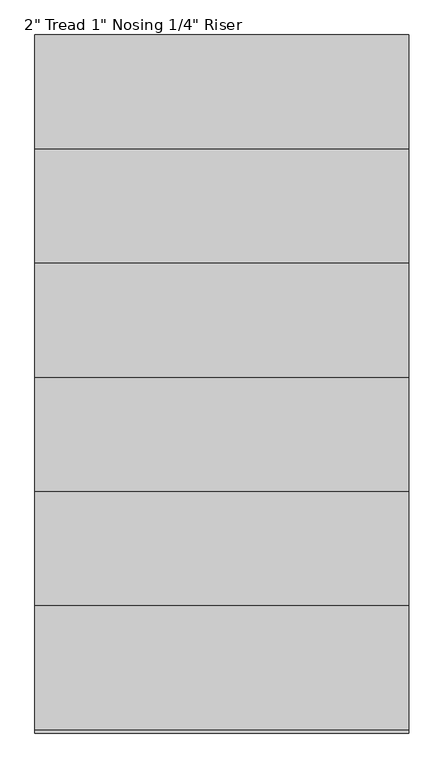
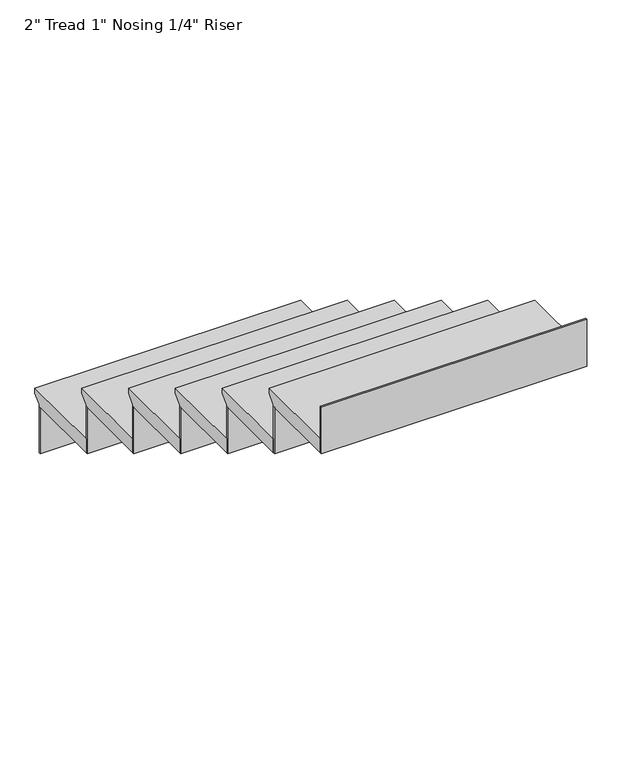
"""IFC4 building model written with IfcOpenShell, lengths in millimetres: stair flight geometry."""

from ifc_helpers import new_model, si_unit, origin, place, context, project, spatial, faceted_brep, source, transform, mapped, element, save


def stair_flight_6c6ed0d7(model_context):
    return source(origin(), model_context, "Body", "Brep", [
        faceted_brep([(-7682.5118598, 4060.7368529, 1335.6166667), (-7682.5118598, 4060.7368529, 1354.6666667), (-6768.1118598, 4060.7368529, 1354.6666667), (-6768.1118598, 4060.7368529, 1335.6166667), (-7682.5118598, 4035.3368529, 1310.2166667), (-6768.1118598, 4035.3368529, 1310.2166667), (-7682.5118598, 3755.9368529, 1354.6666667), (-6768.1118598, 3755.9368529, 1354.6666667), (-6768.1118598, 4035.3368529, 1303.8666667), (-6768.1118598, 3755.9368529, 1303.8666667), (-7682.5118598, 3755.9368529, 1303.8666667), (-7682.5118598, 4035.3368529, 1303.8666667)], [[[0, 1, 2, 3]], [[4, 0, 3, 5]], [[2, 1, 6, 7]], [[8, 9, 10, 11]], [[2, 7, 9, 8, 5, 3]], [[8, 11, 4, 5]], [[6, 1, 0, 4, 11, 10]], [[7, 6, 10, 9]]]),
        faceted_brep([(-7682.5118598, 4035.3368529, 1303.8666667), (-7682.5118598, 4035.3368529, 1134.5333333), (-7682.5118598, 4028.9868529, 1134.5333333), (-7682.5118598, 4028.9868529, 1303.8666667), (-6768.1118598, 4035.3368529, 1303.8666667), (-6768.1118598, 4028.9868529, 1303.8666667), (-6768.1118598, 4028.9868529, 1134.5333333), (-6768.1118598, 4035.3368529, 1134.5333333)], [[[0, 1, 2, 3]], [[4, 5, 6, 7]], [[1, 0, 4, 7]], [[2, 1, 7, 6]], [[3, 2, 6, 5]], [[0, 3, 5, 4]]]),
        faceted_brep([(-7682.5118598, 3755.9368529, 1473.2), (-7682.5118598, 3755.9368529, 1303.8666667), (-7682.5118598, 3749.5868529, 1303.8666667), (-7682.5118598, 3749.5868529, 1473.2), (-6768.1118598, 3755.9368529, 1473.2), (-6768.1118598, 3749.5868529, 1473.2), (-6768.1118598, 3749.5868529, 1303.8666667), (-6768.1118598, 3755.9368529, 1303.8666667)], [[[0, 1, 2, 3]], [[4, 5, 6, 7]], [[1, 0, 4, 7]], [[2, 1, 7, 6]], [[3, 2, 6, 5]], [[0, 3, 5, 4]]]),
        faceted_brep([(-6768.1118598, 3781.3368529, 1524.0), (-7682.5118598, 3781.3368529, 1524.0), (-7682.5118598, 3476.5368529, 1524.0), (-6768.1118598, 3476.5368529, 1524.0), (-6768.1118598, 3755.9368529, 1473.2), (-6768.1118598, 3476.5368529, 1473.2), (-7682.5118598, 3476.5368529, 1473.2), (-7682.5118598, 3755.9368529, 1473.2), (-6768.1118598, 3755.9368529, 1479.55), (-6768.1118598, 3781.3368529, 1504.95), (-7682.5118598, 3755.9368529, 1479.55), (-7682.5118598, 3781.3368529, 1504.95)], [[[0, 1, 2, 3]], [[4, 5, 6, 7]], [[0, 3, 5, 4, 8, 9]], [[4, 7, 10, 8]], [[2, 1, 11, 10, 7, 6]], [[3, 2, 6, 5]], [[11, 1, 0, 9]], [[10, 11, 9, 8]]]),
        faceted_brep([(-7682.5118598, 3476.5368529, 1642.5333333), (-7682.5118598, 3476.5368529, 1473.2), (-7682.5118598, 3470.1868529, 1473.2), (-7682.5118598, 3470.1868529, 1642.5333333), (-6768.1118598, 3476.5368529, 1642.5333333), (-6768.1118598, 3470.1868529, 1642.5333333), (-6768.1118598, 3470.1868529, 1473.2), (-6768.1118598, 3476.5368529, 1473.2)], [[[0, 1, 2, 3]], [[4, 5, 6, 7]], [[1, 0, 4, 7]], [[2, 1, 7, 6]], [[3, 2, 6, 5]], [[0, 3, 5, 4]]]),
        faceted_brep([(-6768.1118598, 3501.9368529, 1693.3333333), (-7682.5118598, 3501.9368529, 1693.3333333), (-7682.5118598, 3197.1368529, 1693.3333333), (-6768.1118598, 3197.1368529, 1693.3333333), (-6768.1118598, 3476.5368529, 1642.5333333), (-6768.1118598, 3197.1368529, 1642.5333333), (-7682.5118598, 3197.1368529, 1642.5333333), (-7682.5118598, 3476.5368529, 1642.5333333), (-6768.1118598, 3476.5368529, 1648.8833333), (-6768.1118598, 3501.9368529, 1674.2833333), (-7682.5118598, 3476.5368529, 1648.8833333), (-7682.5118598, 3501.9368529, 1674.2833333)], [[[0, 1, 2, 3]], [[4, 5, 6, 7]], [[0, 3, 5, 4, 8, 9]], [[4, 7, 10, 8]], [[2, 1, 11, 10, 7, 6]], [[3, 2, 6, 5]], [[11, 1, 0, 9]], [[10, 11, 9, 8]]]),
        faceted_brep([(-7682.5118598, 3197.1368529, 1811.8666667), (-7682.5118598, 3197.1368529, 1642.5333333), (-7682.5118598, 3190.7868529, 1642.5333333), (-7682.5118598, 3190.7868529, 1811.8666667), (-6768.1118598, 3197.1368529, 1811.8666667), (-6768.1118598, 3190.7868529, 1811.8666667), (-6768.1118598, 3190.7868529, 1642.5333333), (-6768.1118598, 3197.1368529, 1642.5333333)], [[[0, 1, 2, 3]], [[4, 5, 6, 7]], [[1, 0, 4, 7]], [[2, 1, 7, 6]], [[3, 2, 6, 5]], [[0, 3, 5, 4]]]),
        faceted_brep([(-6768.1118598, 3222.5368529, 1862.6666667), (-7682.5118598, 3222.5368529, 1862.6666667), (-7682.5118598, 2917.7368529, 1862.6666667), (-6768.1118598, 2917.7368529, 1862.6666667), (-6768.1118598, 3197.1368529, 1811.8666667), (-6768.1118598, 2917.7368529, 1811.8666667), (-7682.5118598, 2917.7368529, 1811.8666667), (-7682.5118598, 3197.1368529, 1811.8666667), (-6768.1118598, 3197.1368529, 1818.2166667), (-6768.1118598, 3222.5368529, 1843.6166667), (-7682.5118598, 3197.1368529, 1818.2166667), (-7682.5118598, 3222.5368529, 1843.6166667)], [[[0, 1, 2, 3]], [[4, 5, 6, 7]], [[0, 3, 5, 4, 8, 9]], [[4, 7, 10, 8]], [[2, 1, 11, 10, 7, 6]], [[3, 2, 6, 5]], [[11, 1, 0, 9]], [[10, 11, 9, 8]]]),
        faceted_brep([(-7682.5118598, 2917.7368529, 1981.2), (-7682.5118598, 2917.7368529, 1811.8666667), (-7682.5118598, 2911.3868529, 1811.8666667), (-7682.5118598, 2911.3868529, 1981.2), (-6768.1118598, 2917.7368529, 1981.2), (-6768.1118598, 2911.3868529, 1981.2), (-6768.1118598, 2911.3868529, 1811.8666667), (-6768.1118598, 2917.7368529, 1811.8666667)], [[[0, 1, 2, 3]], [[4, 5, 6, 7]], [[1, 0, 4, 7]], [[2, 1, 7, 6]], [[3, 2, 6, 5]], [[0, 3, 5, 4]]]),
        faceted_brep([(-6768.1118598, 2943.1368529, 2032.0), (-7682.5118598, 2943.1368529, 2032.0), (-7682.5118598, 2638.3368529, 2032.0), (-6768.1118598, 2638.3368529, 2032.0), (-6768.1118598, 2917.7368529, 1981.2), (-6768.1118598, 2638.3368529, 1981.2), (-7682.5118598, 2638.3368529, 1981.2), (-7682.5118598, 2917.7368529, 1981.2), (-6768.1118598, 2917.7368529, 1987.55), (-6768.1118598, 2943.1368529, 2012.95), (-7682.5118598, 2917.7368529, 1987.55), (-7682.5118598, 2943.1368529, 2012.95)], [[[0, 1, 2, 3]], [[4, 5, 6, 7]], [[0, 3, 5, 4, 8, 9]], [[4, 7, 10, 8]], [[2, 1, 11, 10, 7, 6]], [[3, 2, 6, 5]], [[11, 1, 0, 9]], [[10, 11, 9, 8]]]),
        faceted_brep([(-7682.5118598, 2358.9368529, 2319.8666667), (-7682.5118598, 2358.9368529, 2150.5333333), (-7682.5118598, 2352.5868529, 2150.5333333), (-7682.5118598, 2352.5868529, 2319.8666667), (-6768.1118598, 2358.9368529, 2319.8666667), (-6768.1118598, 2352.5868529, 2319.8666667), (-6768.1118598, 2352.5868529, 2150.5333333), (-6768.1118598, 2358.9368529, 2150.5333333)], [[[0, 1, 2, 3]], [[4, 5, 6, 7]], [[1, 0, 4, 7]], [[2, 1, 7, 6]], [[3, 2, 6, 5]], [[0, 3, 5, 4]]]),
        faceted_brep([(-7682.5118598, 2638.3368529, 2150.5333333), (-7682.5118598, 2638.3368529, 1981.2), (-7682.5118598, 2631.9868529, 1981.2), (-7682.5118598, 2631.9868529, 2150.5333333), (-6768.1118598, 2638.3368529, 2150.5333333), (-6768.1118598, 2631.9868529, 2150.5333333), (-6768.1118598, 2631.9868529, 1981.2), (-6768.1118598, 2638.3368529, 1981.2)], [[[0, 1, 2, 3]], [[4, 5, 6, 7]], [[1, 0, 4, 7]], [[2, 1, 7, 6]], [[3, 2, 6, 5]], [[0, 3, 5, 4]]]),
        faceted_brep([(-6768.1118598, 2358.9368529, 2201.3333333), (-6768.1118598, 2384.3368529, 2201.3333333), (-6768.1118598, 2663.7368529, 2201.3333333), (-7682.5118598, 2663.7368529, 2201.3333333), (-7682.5118598, 2358.9368529, 2201.3333333), (-6768.1118598, 2384.3368529, 2150.5333333), (-6768.1118598, 2358.9368529, 2150.5333333), (-7682.5118598, 2358.9368529, 2150.5333333), (-7682.5118598, 2638.3368529, 2150.5333333), (-6768.1118598, 2638.3368529, 2150.5333333), (-6768.1118598, 2638.3368529, 2156.8833333), (-6768.1118598, 2663.7368529, 2182.2833333), (-7682.5118598, 2638.3368529, 2156.8833333), (-7682.5118598, 2663.7368529, 2182.2833333)], [[[0, 1, 2, 3, 4]], [[5, 6, 7, 8, 9]], [[1, 0, 6, 5]], [[2, 1, 5, 9, 10, 11]], [[9, 8, 12, 10]], [[4, 3, 13, 12, 8, 7]], [[0, 4, 7, 6]], [[13, 3, 2, 11]], [[12, 13, 11, 10]]]),
    ])


if __name__ == "__main__":
    model = new_model("IFC4")
    model_context = context("Model", 3, world=origin())
    ifc_project = project(units=[si_unit("LENGTHUNIT", "METRE", prefix="MILLI")], contexts=[model_context])
    site = spatial("IfcSite", under=ifc_project)
    building = spatial("IfcBuilding", under=site)
    placement = place(None, origin())
    stair_flight_shape = stair_flight_6c6ed0d7(model_context)
    element("IfcStairFlight", 1, ObjectType="2\" Tread 1\" Nosing 1/4\" Riser", at=placement, inside=building, context=model_context, shape_type="MappedRepresentation", body=[
        mapped(stair_flight_shape, transform((0.0, 0.0, 0.0), x_axis=(1.0, 0.0, 0.0), y_axis=(0.0, 1.0, 0.0), z_axis=(0.0, 0.0, 1.0))),
    ])
    save(model, "model.ifc")
